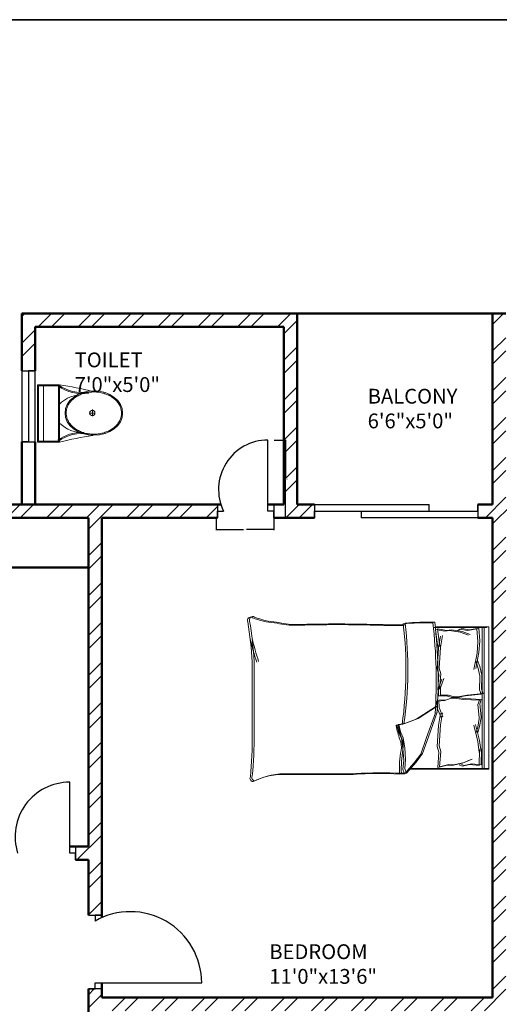
# Model space of a CAD drawing. Units: inches. Extents: x 963 to 2075, y 289 to 2657.
# Tile 81 of 98: x 1349 to 1511, y 2325 to 2657. Entities that reach past the tile are written whole.
import ezdxf

# ---------------------------------------------------------------- set-up
doc = ezdxf.new("R2010")
doc.units = ezdxf.units.IN
for name, color, linetype, lineweight in [('A-ANNO-DIMS', 2, 'Continuous', 18), ('A-ANNO-TTLB', 7, 'Continuous', 35), ('A-AREA-IDEN', 7, 'Continuous', 18), ('A-DOOR', 4, 'Continuous', 25), ('A-FLOR-FIXT', 9, 'Continuous', 18), ('A-FURN', 8, 'Continuous', 18), ('A-GLAZ', 3, 'Continuous', 25), ('A-WALL', 7, 'Continuous', 50), ('A-WALL-PATT', 8, 'Continuous', 13)]:
    doc.layers.add(name, color=color, linetype=linetype, lineweight=lineweight)
doc.styles.get("Standard").update_dxf_attribs({"font": 'arial.ttf'})
doc.dimstyles.get("Standard").update_dxf_attribs({"dimtxt": 0.18, "dimasz": 0.18, "dimexe": 0.18, "dimexo": 0.0625, "dimgap": 0.09, "dimtad": 0, "dimtih": 1, "dimtoh": 1, "dimdec": 4, "dimzin": 0, "dimdsep": 46, "dimtxsty": 'Standard', "dimcen": 0.09, "dimadec": 0, "dimazin": 0, "dimtfac": 1, "dimtdec": 4, "dimtofl": 0, "dimtmove": 0, "dimatfit": 3, "dimfxl": 1, "dimtolj": 1, "dimtzin": 0, "dimarcsym": 0})

# ---------------------------------------------------------------- blocks, each defined once
blk = doc.blocks.new('A$C31115884')
for p, q in [((283.1, 497.7), (223.4, 497.7)), ((257.5, 466.4), (257.5, 523.2)), ((0, 200), (0, 0)), ((520, 200), (0, 200)), ((10, 190), (10, 10)), ((510, 190), (10, 190)), ((510, 10), (510, 190)), ((520, 0), (520, 200)), ((510, 54.5), (0, 54.5)), ((10, 10), (510, 10)), ((0, 0), (520, 0))]:
    blk.add_line(p, q)
blk.add_circle((255.6, 496.4), 23.6)
for centre, radius, start, end in [((2777.7, -204.6), 2807, 165.4549, 171.71327), ((-294.5, 403.3), 364.7, 324.20913, 9.34987), ((-294.5, 403.3), 374.7, 324.20913, 9.34987), ((805.8, 403.3), 364.7, 170.65013, 215.79087), ((3237, 905), 2807, 188.28673, 194.5451), ((139.5, 406.2), 293.5, 315.84364, 2.65635), ((805.8, 403.3), 374.7, 179.20365, 215.79087), ((383.6, 406.2), 293.5, 190.27735, 224.15636)]:
    blk.add_arc(centre, radius, start, end)
blk.add_ellipse((256.2, 509.9), major_axis=(0, -260.7), ratio=0.772727)
blk.add_open_spline([(256.2, 259.2), (263.1, 259.2), (270, 259.7), (287.8, 262.3), (298.7, 265.1), (319.9, 273.1), (330.2, 278.4), (350.1, 291.1), (359.7, 298.7), (377.7, 315.9), (386.2, 325.5), (401.7, 346.6), (408.8, 358.1), (421.3, 382.5), (426.8, 395.5), (435.9, 422.4), (439.5, 436.4), (444.8, 465.1), (446.5, 479.7), (447.9, 509.2), (447.6, 524), (445, 553.3), (442.7, 567.8), (436.3, 596), (432.1, 609.7), (421.9, 636), (416, 648.6), (402.5, 672.1), (395, 683), (378.6, 703), (369.8, 712.1), (351.1, 728), (341.3, 734.8), (320.9, 746.2), (310.4, 750.7), (288.9, 757.3), (278, 759.4), (256, 761), (245, 760.6), (223.1, 757.2), (212.3, 754.3), (191.1, 746.1), (180.8, 740.7), (160.9, 727.8), (151.4, 720.1), (133.5, 702.7), (125.1, 693), (109.6, 671.7), (102.6, 660.2), (90.2, 635.7), (84.9, 622.7), (76, 595.6), (72.4, 581.6), (67.2, 552.9), (65.6, 538.2), (64.4, 508.8), (64.8, 494), (67.5, 464.7), (69.9, 450.2), (76.6, 422), (80.8, 408.3), (91.1, 382.2), (97.2, 369.7), (110.8, 346.3), (118.4, 335.4), (134.8, 315.6), (143.7, 306.7), (162.4, 290.9), (172.3, 284.2), (192.8, 273), (203.3, 268.6), (224.8, 262.2), (235.8, 260.2), (249.9, 259.3), (253, 259.2), (256.2, 259.2)], degree=3, knots=[0, 0, 0, 0, 0.110105, 0.110105, 0.285049, 0.285049, 0.459994, 0.459994, 0.634938, 0.634938, 0.809882, 0.809882, 0.984827, 0.984827, 1.159771, 1.159771, 1.334715, 1.334715, 1.50966, 1.50966, 1.684604, 1.684604, 1.859549, 1.859549, 2.034493, 2.034493, 2.209437, 2.209437, 2.384382, 2.384382, 2.559326, 2.559326, 2.73427, 2.73427, 2.909215, 2.909215, 3.084159, 3.084159, 3.259103, 3.259103, 3.434048, 3.434048, 3.608992, 3.608992, 3.783936, 3.783936, 3.958881, 3.958881, 4.133825, 4.133825, 4.30877, 4.30877, 4.483714, 4.483714, 4.658658, 4.658658, 4.833603, 4.833603, 5.008547, 5.008547, 5.183491, 5.183491, 5.358436, 5.358436, 5.53338, 5.53338, 5.708324, 5.708324, 5.883269, 5.883269, 6.058213, 6.058213, 6.233158, 6.233158, 6.283185, 6.283185, 6.283185, 6.283185])
blk = doc.blocks.new('BED-DOUBLE')
for p, q in [((1236.12, 2450.52), (1254.23, 2450.52)), ((1236.12, 2450.52), (1254.23, 2450.52)), ((1236.76, 2450.75), (1254.87, 2450.75)), ((1236.76, 2450.75), (1254.87, 2450.75)), ((1238.25, 2444.94), (1237.53, 2450.04)), ((1237.53, 2450.04), (1240.71, 2449.46)), ((1238.25, 2444.94), (1237.53, 2450.04)), ((1237.53, 2450.04), (1240.71, 2449.46)), ((1245.77, 2450.18), (1244.76, 2449.61)), ((1245.77, 2450.18), (1244.76, 2449.61)), ((1248.37, 2449.75), (1245.77, 2450.18)), ((1248.37, 2449.75), (1245.77, 2450.18)), ((1250.92, 2450.1), (1247.74, 2449.52)), ((1250.92, 2450.1), (1247.74, 2449.52)), ((1251.56, 2450.33), (1248.37, 2449.75)), ((1251.56, 2450.33), (1248.37, 2449.75)), ((1250.89, 2450.1), (1251.22, 2445.82)), ((1250.89, 2450.1), (1251.22, 2445.82)), ((1251.53, 2450.32), (1251.86, 2446.04)), ((1251.53, 2450.32), (1251.86, 2446.04)), ((1252.7, 2450.52), (1252.7, 2402.73)), ((1252.7, 2450.52), (1252.7, 2402.73)), ((1253.34, 2450.75), (1253.34, 2402.96)), ((1253.34, 2450.75), (1253.34, 2402.96)), ((1254.87, 2450.75), (1254.87, 2402.73)), ((1237.61, 2444.71), (1236.89, 2449.81)), ((1236.89, 2449.81), (1240.07, 2449.23)), ((1237.61, 2444.71), (1236.89, 2449.81)), ((1236.89, 2449.81), (1240.07, 2449.23)), ((1238.6, 2447.61), (1237.94, 2443.58)), ((1238.6, 2447.61), (1237.94, 2443.58)), ((1239.24, 2447.84), (1238.58, 2443.81)), ((1239.24, 2447.84), (1238.58, 2443.81)), ((1240.07, 2449.23), (1241.66, 2449.52)), ((1240.07, 2449.23), (1241.66, 2449.52)), ((1240.71, 2449.46), (1242.3, 2449.75)), ((1240.71, 2449.46), (1242.3, 2449.75)), ((1241.66, 2449.52), (1245.28, 2448.94)), ((1241.66, 2449.52), (1245.28, 2448.94)), ((1242.3, 2449.75), (1245.92, 2449.17)), ((1242.3, 2449.75), (1245.92, 2449.17)), ((1245.13, 2449.96), (1244.12, 2449.38)), ((1245.13, 2449.96), (1244.12, 2449.38)), ((1247.74, 2449.52), (1245.13, 2449.96)), ((1247.74, 2449.52), (1245.13, 2449.96)), ((1245.28, 2448.94), (1248.02, 2447.93)), ((1245.28, 2448.94), (1248.02, 2447.93)), ((1245.92, 2449.17), (1248.66, 2448.16)), ((1245.92, 2449.17), (1248.66, 2448.16)), ((1237.94, 2443.58), (1237.51, 2436.57)), ((1237.94, 2443.58), (1237.51, 2436.57)), ((1237.94, 2443.58), (1237.61, 2444.71)), ((1237.94, 2443.58), (1237.61, 2444.71)), ((1238.58, 2443.81), (1238.15, 2436.8)), ((1238.58, 2443.81), (1238.15, 2436.8)), ((1238.58, 2443.81), (1238.25, 2444.94)), ((1238.58, 2443.81), (1238.25, 2444.94)), ((1251.21, 2445.71), (1250.92, 2441.89)), ((1251.21, 2445.71), (1250.92, 2441.89)), ((1251.22, 2445.82), (1251.21, 2445.71)), ((1251.22, 2445.82), (1251.21, 2445.71)), ((1251.84, 2445.94), (1251.56, 2442.11)), ((1251.84, 2445.94), (1251.56, 2442.11)), ((1251.86, 2446.04), (1251.84, 2445.94)), ((1251.86, 2446.04), (1251.84, 2445.94)), ((1250.92, 2441.89), (1249.9, 2436.39)), ((1250.92, 2441.89), (1249.9, 2436.39)), ((1251.56, 2442.11), (1250.54, 2436.62)), ((1251.56, 2442.11), (1250.54, 2436.62)), ((1174.99, 2438.93), (1174.99, 2414.32)), ((1174.99, 2438.93), (1174.99, 2414.32)), ((1175.63, 2439.16), (1175.63, 2414.55)), ((1175.63, 2439.16), (1175.63, 2414.55)), ((1238.15, 2436.8), (1238.7, 2434.84)), ((1238.15, 2436.8), (1238.7, 2434.84)), ((1250.48, 2439.14), (1251.21, 2437.12)), ((1250.48, 2439.14), (1251.21, 2437.12)), ((1251.12, 2439.37), (1251.84, 2437.34)), ((1251.12, 2439.37), (1251.84, 2437.34)), ((1251.21, 2437.12), (1251.93, 2434.22)), ((1251.21, 2437.12), (1251.93, 2434.23)), ((1251.84, 2437.34), (1252.57, 2434.45)), ((1251.84, 2437.34), (1252.57, 2434.45)), ((1237.51, 2436.57), (1238.06, 2434.61)), ((1237.51, 2436.57), (1238.06, 2434.61)), ((1238.06, 2434.61), (1237.66, 2429.48)), ((1238.06, 2434.61), (1237.66, 2429.48)), ((1238.7, 2434.84), (1238.3, 2429.71)), ((1238.7, 2434.84), (1238.3, 2429.71)), ((1251.93, 2433.9), (1251.78, 2429.46)), ((1251.93, 2433.9), (1251.78, 2429.46)), ((1251.93, 2434.23), (1251.93, 2433.9)), ((1251.93, 2434.22), (1251.93, 2433.9)), ((1252.57, 2434.13), (1252.42, 2429.69)), ((1252.57, 2434.13), (1252.42, 2429.69)), ((1252.57, 2434.45), (1252.57, 2434.13)), ((1252.57, 2434.45), (1252.57, 2434.13)), ((1237.97, 2429.89), (1239.06, 2433.04)), ((1237.97, 2429.89), (1239.06, 2433.04)), ((1238.61, 2430.12), (1239.7, 2433.26)), ((1238.61, 2430.12), (1239.7, 2433.26)), ((1238.61, 2427.66), (1238.61, 2430.12)), ((1238.61, 2427.66), (1238.61, 2430.12)), ((1237.97, 2427.43), (1237.97, 2429.89)), ((1237.97, 2427.43), (1237.97, 2429.89)), ((1240.65, 2427.43), (1237.97, 2427.43)), ((1240.65, 2427.43), (1237.97, 2427.43)), ((1241.29, 2427.66), (1238.61, 2427.66)), ((1241.29, 2427.66), (1238.61, 2427.66)), ((1242.53, 2426.86), (1240.65, 2427.43)), ((1242.53, 2426.86), (1240.65, 2427.43)), ((1242.49, 2426.79), (1240.66, 2426.09)), ((1242.49, 2426.79), (1240.66, 2426.09)), ((1243.17, 2427.08), (1241.29, 2427.66)), ((1243.17, 2427.08), (1241.29, 2427.66)), ((1243.79, 2426.87), (1242.49, 2426.79)), ((1243.79, 2426.87), (1242.49, 2426.79)), ((1243.83, 2426.86), (1242.53, 2426.86)), ((1243.83, 2426.86), (1242.53, 2426.86)), ((1244.47, 2427.08), (1243.17, 2427.08)), ((1244.47, 2427.08), (1243.17, 2427.08)), ((1247, 2426.49), (1243.79, 2426.87)), ((1247, 2426.49), (1243.79, 2426.87)), ((1247.01, 2427.43), (1243.83, 2426.86)), ((1247.01, 2427.43), (1243.83, 2426.86)), ((1247.65, 2427.66), (1244.47, 2427.08)), ((1247.65, 2427.66), (1244.47, 2427.08)), ((1252.36, 2428.01), (1247.01, 2427.43)), ((1252.36, 2428.01), (1247.01, 2427.43)), ((1253, 2428.24), (1247.65, 2427.66)), ((1253, 2428.24), (1247.65, 2427.66)), ((1251.78, 2429.46), (1252.36, 2428.01)), ((1251.78, 2429.46), (1252.36, 2428.01)), ((1252.42, 2429.69), (1253, 2428.24)), ((1252.42, 2429.69), (1253, 2428.24)), ((1236.85, 2423.74), (1230.36, 2419.55)), ((1236.85, 2423.74), (1230.36, 2419.55)), ((1237.49, 2423.96), (1231, 2419.77)), ((1237.49, 2423.96), (1231, 2419.77)), ((1240.02, 2425.86), (1237.34, 2425.7)), ((1240.02, 2425.86), (1237.34, 2425.7)), ((1237.34, 2425.7), (1237.49, 2423.24)), ((1237.34, 2425.7), (1237.49, 2423.24)), ((1240.66, 2426.09), (1237.98, 2425.93)), ((1240.66, 2426.09), (1237.98, 2425.93)), ((1237.98, 2425.93), (1238.13, 2423.47)), ((1237.98, 2425.93), (1238.13, 2423.47)), ((1238.13, 2423.47), (1239.42, 2420.4)), ((1238.13, 2423.47), (1239.42, 2420.4)), ((1241.86, 2426.56), (1240.02, 2425.86)), ((1241.86, 2426.56), (1240.02, 2425.86)), ((1243.15, 2426.64), (1241.86, 2426.56)), ((1243.15, 2426.64), (1241.86, 2426.56)), ((1246.37, 2426.26), (1243.15, 2426.64)), ((1246.37, 2426.26), (1243.15, 2426.64)), ((1251.74, 2426.02), (1246.37, 2426.26)), ((1251.74, 2426.02), (1246.37, 2426.26)), ((1252.38, 2426.25), (1247, 2426.49)), ((1252.38, 2426.25), (1247, 2426.49)), ((1251.25, 2424.54), (1251.74, 2426.02)), ((1251.25, 2424.54), (1251.74, 2426.02)), ((1251.68, 2420.11), (1251.25, 2424.54)), ((1251.68, 2420.11), (1251.25, 2424.54)), ((1251.89, 2424.77), (1252.38, 2426.25)), ((1251.89, 2424.77), (1252.38, 2426.25)), ((1252.31, 2420.34), (1251.89, 2424.77)), ((1252.31, 2420.34), (1251.89, 2424.77)), ((1233.92, 2413.35), (1236.85, 2421.69)), ((1233.92, 2413.35), (1236.85, 2421.69)), ((1234.56, 2413.58), (1237.49, 2421.92)), ((1234.56, 2413.58), (1237.49, 2421.92)), ((1237.49, 2423.24), (1238.78, 2420.17)), ((1237.49, 2423.24), (1238.78, 2420.17)), ((1238.6, 2421.43), (1237.94, 2417.4)), ((1238.6, 2421.43), (1237.94, 2417.4)), ((1239.24, 2421.66), (1238.58, 2417.63)), ((1239.24, 2421.66), (1238.58, 2417.63)), ((1251.7, 2419.79), (1251.68, 2420.11)), ((1251.7, 2419.79), (1251.68, 2420.11)), ((1252.33, 2420.02), (1252.31, 2420.34)), ((1252.33, 2420.02), (1252.31, 2420.34)), ((1225.87, 2417.84), (1223.86, 2417.53)), ((1225.87, 2417.84), (1223.86, 2417.53)), ((1223.86, 2417.53), (1224.47, 2415.05)), ((1223.86, 2417.53), (1224.47, 2415.05)), ((1226.51, 2418.07), (1224.49, 2417.76)), ((1226.51, 2418.07), (1224.49, 2417.76)), ((1224.49, 2417.76), (1225.11, 2415.28)), ((1224.49, 2417.76), (1225.11, 2415.28)), ((1230.36, 2419.55), (1225.87, 2417.84)), ((1230.36, 2419.55), (1225.87, 2417.84)), ((1231, 2419.77), (1226.51, 2418.07)), ((1231, 2419.77), (1226.51, 2418.07)), ((1237.94, 2417.4), (1237.51, 2410.39)), ((1237.94, 2417.4), (1237.51, 2410.39)), ((1238.58, 2417.63), (1238.15, 2410.62)), ((1238.58, 2417.63), (1238.15, 2410.62)), ((1251.16, 2412.08), (1249.81, 2417.5)), ((1251.16, 2412.08), (1249.81, 2417.5)), ((1251.8, 2412.31), (1250.45, 2417.73)), ((1251.8, 2412.31), (1250.45, 2417.73)), ((1250.56, 2414.79), (1251.15, 2416.86)), ((1250.56, 2414.79), (1251.15, 2416.86)), ((1251.15, 2416.86), (1251.7, 2419.79)), ((1251.15, 2416.86), (1251.7, 2419.79)), ((1251.2, 2415.02), (1251.79, 2417.09)), ((1251.2, 2415.02), (1251.79, 2417.09)), ((1251.79, 2417.09), (1252.33, 2420.02)), ((1251.79, 2417.09), (1252.33, 2420.02)), ((1224.47, 2415.05), (1225.4, 2413.04)), ((1224.47, 2415.05), (1225.4, 2413.04)), ((1225.11, 2415.28), (1226.04, 2413.27)), ((1225.11, 2415.28), (1226.04, 2413.27)), ((1232.54, 2408), (1234.56, 2413.58)), ((1232.54, 2408), (1234.56, 2413.58)), ((1225.4, 2413.04), (1225.87, 2409.63)), ((1225.4, 2413.04), (1225.87, 2409.63)), ((1226.04, 2413.27), (1226.51, 2409.86)), ((1226.04, 2413.27), (1226.51, 2409.86)), ((1231.9, 2407.77), (1233.92, 2413.35)), ((1231.9, 2407.78), (1233.92, 2413.35)), ((1237.51, 2410.39), (1238.06, 2408.43)), ((1237.51, 2410.39), (1238.06, 2408.43)), ((1238.15, 2410.62), (1238.7, 2408.66)), ((1238.15, 2410.62), (1238.7, 2408.66)), ((1251.69, 2408.28), (1251.16, 2412.08)), ((1251.69, 2408.28), (1251.16, 2412.08)), ((1252.33, 2408.51), (1251.8, 2412.31)), ((1252.33, 2408.51), (1251.8, 2412.31)), ((1225.87, 2409.63), (1226.18, 2405.76)), ((1225.87, 2409.63), (1226.18, 2405.76)), ((1226.51, 2409.86), (1226.82, 2405.99)), ((1226.51, 2409.86), (1226.82, 2405.99)), ((1229.74, 2404.83), (1231.9, 2407.78)), ((1229.74, 2404.83), (1231.9, 2407.77)), ((1230.38, 2405.06), (1232.54, 2408)), ((1230.38, 2405.06), (1232.54, 2408)), ((1238.06, 2408.43), (1237.66, 2403.3)), ((1238.06, 2408.43), (1237.66, 2403.3)), ((1238.7, 2408.66), (1238.3, 2403.52)), ((1238.7, 2408.66), (1238.3, 2403.52)), ((1251.68, 2403.88), (1251.77, 2409.29)), ((1251.68, 2403.88), (1251.77, 2409.28)), ((1251.77, 2409.29), (1251.69, 2408.28)), ((1251.77, 2409.28), (1251.69, 2408.28)), ((1252.31, 2404.11), (1252.41, 2409.51)), ((1252.31, 2404.11), (1252.41, 2409.51)), ((1252.41, 2409.51), (1252.33, 2408.51)), ((1252.41, 2409.51), (1252.33, 2408.51)), ((1226.18, 2405.76), (1225.87, 2402.66)), ((1226.18, 2405.76), (1225.87, 2402.66)), ((1226.49, 2401.13), (1229.74, 2404.83)), ((1226.49, 2401.13), (1229.74, 2404.83)), ((1226.82, 2405.99), (1226.51, 2402.89)), ((1226.82, 2405.99), (1226.51, 2402.89)), ((1227.13, 2401.36), (1230.38, 2405.06)), ((1227.13, 2401.36), (1230.38, 2405.06)), ((1237.66, 2403.3), (1240.8, 2404.07)), ((1237.66, 2403.3), (1240.8, 2404.07)), ((1238.3, 2403.52), (1241.44, 2404.3)), ((1238.3, 2403.52), (1241.44, 2404.3)), ((1240.8, 2404.07), (1242.4, 2403.88)), ((1240.8, 2404.07), (1242.4, 2403.88)), ((1241.44, 2404.3), (1243.04, 2404.11)), ((1241.44, 2404.3), (1243.04, 2404.11)), ((1242.4, 2403.88), (1245.98, 2404.69)), ((1242.4, 2403.88), (1245.98, 2404.69)), ((1243.04, 2404.11), (1246.61, 2404.91)), ((1243.04, 2404.11), (1246.61, 2404.91)), ((1245.89, 2403.67), (1244.85, 2404.18)), ((1245.89, 2403.67), (1244.85, 2404.18)), ((1246.53, 2403.89), (1245.49, 2404.41)), ((1246.53, 2403.89), (1245.49, 2404.41)), ((1248.46, 2404.26), (1245.89, 2403.67)), ((1248.46, 2404.26), (1245.89, 2403.67)), ((1245.98, 2404.69), (1248.65, 2405.87)), ((1245.98, 2404.69), (1248.65, 2405.87)), ((1249.1, 2404.49), (1246.53, 2403.89)), ((1249.1, 2404.49), (1246.53, 2403.89)), ((1246.61, 2404.91), (1249.29, 2406.1)), ((1246.61, 2404.91), (1249.29, 2406.09)), ((1251.68, 2403.88), (1248.46, 2404.26)), ((1251.68, 2403.88), (1248.46, 2404.26)), ((1252.31, 2404.11), (1249.1, 2404.49)), ((1252.31, 2404.11), (1249.1, 2404.49)), ((1224.74, 2401.05), (1226.49, 2401.13, 3.87)), ((1224.74, 2401.05), (1226.49, 2401.13, 3.87)), ((1225.38, 2401.28), (1227.13, 2401.36, 3.87)), ((1225.38, 2401.28), (1227.13, 2401.36, 3.87)), ((1225.87, 2402.66), (1226.49, 2401.13)), ((1225.87, 2402.66), (1226.49, 2401.13)), ((1226.51, 2402.89), (1227.13, 2401.36)), ((1226.51, 2402.89), (1227.13, 2401.36)), ((1254.23, 2402.73), (1227.62, 2402.73)), ((1254.23, 2402.73), (1227.62, 2402.73)), ((1254.87, 2402.96), (1228.26, 2402.96)), ((1254.87, 2402.96), (1228.26, 2402.96)), ((1254.87, 2402.73), (1254.23, 2402.73))]:
    blk.add_line(p, q)
for centre, radius, start, end in [((1174.51, 2452.91), 1.09, 56.1736, 203.4781), ((1174.51, 2452.91), 1.09, 56.1736, 203.4781), ((1175.15, 2453.14), 1.09, 56.1736, 203.4781), ((1175.15, 2453.14), 1.09, 56.1736, 203.4781), ((1183.96, 2475.65), 23.56, 247.9751, 266.652), ((1183.96, 2475.65), 23.56, 247.9751, 266.652), ((1184.6, 2475.88), 23.56, 247.9751, 266.652), ((1184.6, 2475.88), 23.56, 247.9751, 266.652), ((1053.4, 2432.57), 121.76, 2.9958, 9.4091), ((1053.4, 2432.57), 121.76, 2.9958, 9.4091), ((1054.03, 2432.8), 121.76, 2.9958, 9.4091), ((1054.03, 2432.8), 121.76, 2.9958, 9.4091), ((1189.72, 2480.89), 29.63, 256.0648, 268.9113), ((1189.72, 2480.89), 29.63, 256.0648, 268.9113), ((1190.36, 2481.12), 29.63, 256.0648, 268.9113), ((1190.36, 2481.12), 29.63, 256.0648, 268.9113), ((1203.62, 1969.17), 482.31, 88.2277, 91.7185), ((1203.62, 1969.17), 482.31, 88.2277, 91.7185), ((1204.26, 1969.4), 482.31, 88.2277, 91.7185), ((1204.26, 1969.4), 482.31, 88.2277, 91.7185), ((1223.06, 2621.3), 170.11, 268.4762, 271.0082), ((1223.06, 2621.3), 170.11, 268.4762, 271.0082), ((1223.7, 2621.53), 170.11, 268.4762, 271.0082), ((1223.7, 2621.53), 170.11, 268.4762, 271.0082), ((1097.92, 2436.24), 129.02, 351.7845, 6.9006), ((1097.92, 2436.24), 129.02, 351.7845, 6.9006), ((1234.14, 2368.83), 83.31, 88.7218, 95.604), ((1234.14, 2368.83), 83.31, 88.7218, 95.604), ((1098.56, 2436.47), 129.02, 351.7845, 6.9006), ((1098.56, 2436.47), 129.02, 351.7845, 6.9006), ((1234.78, 2369.06), 83.31, 88.7218, 95.604), ((1234.78, 2369.06), 83.31, 88.7218, 95.604), ((1072.18, 2432.64), 164.97, 356.0865, 6.7821), ((1072.18, 2432.64), 164.97, 356.0865, 6.7821), ((1072.82, 2432.86), 164.97, 356.0865, 6.7821), ((1072.82, 2432.86), 164.97, 356.0865, 6.7821), ((1278.58, 2471.44), 106.46, 193.3832, 197.7053), ((1278.58, 2471.44), 106.46, 193.3832, 197.7053), ((1277.94, 2471.22), 106.46, 193.3832, 197.7053), ((1277.94, 2471.22), 106.46, 193.3832, 197.7053), ((1223.79, 2417.36), 0.185, 70.2464, 181.1377), ((1223.79, 2417.36), 0.185, 70.2464, 181.1377), ((1252.75, 2422.84), 29.65, 190.6617, 199.8806), ((1252.75, 2422.84), 29.65, 190.6617, 199.8806), ((1224.43, 2417.59), 0.185, 70.2464, 181.1377), ((1224.43, 2417.59), 0.185, 70.2464, 181.1377), ((1253.39, 2423.07), 29.65, 190.6617, 199.8806), ((1253.39, 2423.07), 29.65, 190.6617, 199.8806), ((1041.96, 2412.84), 133.04, 354.4998, 0.6351), ((1041.96, 2412.84), 133.04, 354.4998, 0.6351), ((1042.6, 2413.07), 133.04, 354.4998, 0.6351), ((1042.6, 2413.07), 133.04, 354.4998, 0.6351), ((1219.17, 2410.25), 6.22, 348.6608, 23.7384), ((1219.17, 2410.25), 6.22, 348.6608, 23.7384), ((1219.81, 2410.48), 6.22, 348.6608, 23.7384), ((1219.81, 2410.48), 6.22, 348.6608, 23.7384), ((1260.89, 2402.67), 36.18, 169.8763, 182.5657), ((1260.89, 2402.67), 36.18, 169.8763, 182.5657), ((1261.53, 2402.9), 36.18, 169.8763, 182.5657), ((1261.53, 2402.9), 36.18, 169.8763, 182.5657), ((1176, 2399.81), 1.1, 152.6588, 266.02), ((1176, 2399.81), 1.1, 152.6588, 266.02), ((1185.57, 2377.84), 23.07, 87.4714, 116.4681), ((1185.57, 2377.84), 23.07, 87.4714, 116.4681), ((1186.21, 2378.07), 23.07, 87.4714, 116.4681), ((1186.21, 2378.07), 23.07, 87.4714, 116.4681), ((1186.41, 6962.74), 4561.86, 270.00217, 270.28689), ((1186.41, 6962.74), 4561.86, 270.00217, 270.28689), ((1187.05, 6962.97), 4561.86, 270.00217, 270.28689), ((1187.05, 6962.97), 4561.86, 270.00217, 270.28689), ((1217.92, 2271.73), 129.5, 86.9791, 93.8365), ((1217.92, 2271.73), 129.5, 86.9791, 93.8365), ((1218.56, 2271.96), 129.5, 86.9791, 93.8365), ((1218.56, 2271.96), 129.5, 86.9791, 93.8365), ((1175.36, 2399.58), 1.1, 152.6588, 266.02), ((1175.36, 2399.58), 1.1, 152.6588, 266.02)]:
    blk.add_arc(centre, radius, start, end)
blk = doc.blocks.new('DOOR-4')
for p, q in [((16.99, 2.25), (16.99, 26.25)), ((0, 4.5), (0, 0)), ((18.99, 4.5), (18.99, 0)), ((0, 0), (0, 2.25)), ((0, 2.25), (2, 2.25)), ((18.99, 2.25), (16.99, 2.25)), ((18.99, 0), (18.99, 2.25))]:
    blk.add_line(p, q)
blk.add_arc((16.99, 9.57), 16.68, 90, 206.0308)
blk = doc.blocks.new('*D36')
at = {"layer": 'A-ANNO-DIMS', "color": 0, "lineweight": -2, "transparency": 16777216}
for p, q in [((1434.6, 2515.57), (1438.66, 2515.57)), ((1438.48, 2515.39), (1438.48, 2502.63)), ((1438.48, 2489.5), (1438.48, 2502.26)), ((1434.6, 2489.32), (1438.66, 2489.32))]:
    blk.add_line(p, q, dxfattribs=at)
at = {"layer": 'A-ANNO-DIMS', "color": 0, "transparency": 16777216}
for points in [[(1438.45, 2515.39), (1438.51, 2515.39), (1438.48, 2515.57)], [(1438.45, 2489.5), (1438.51, 2489.5), (1438.48, 2489.32)]]:
    blk.add_solid(points, dxfattribs=at)
at = {"layer": 'Defpoints', "color": 0, "transparency": 16777216}
for p in [(1434.54, 2515.57), (1438.48, 2515.57), (1434.54, 2489.32)]:
    blk.add_point(p, dxfattribs=at)
at = {"layer": 'A-ANNO-DIMS', "color": 0, "transparency": 16777216, "insert": (1438.48, 2502.44), "char_height": 0.18, "attachment_point": 5}
blk.add_mtext('\\A1;DOOR D4 26 TYP.', dxfattribs=at)
blk = doc.blocks.new('*D37')
at = {"layer": 'A-ANNO-DIMS', "color": 0, "lineweight": -2, "transparency": 16777216}
for p, q in [((1415.03, 2489.26), (1415.03, 2485.2)), ((1434.54, 2489.26), (1434.54, 2485.2)), ((1415.21, 2485.38), (1424.26, 2485.38)), ((1434.36, 2485.38), (1425.32, 2485.38))]:
    blk.add_line(p, q, dxfattribs=at)
at = {"layer": 'A-ANNO-DIMS', "color": 0, "transparency": 16777216}
for points in [[(1415.21, 2485.41), (1415.21, 2485.35), (1415.03, 2485.38)], [(1434.36, 2485.41), (1434.36, 2485.35), (1434.54, 2485.38)]]:
    blk.add_solid(points, dxfattribs=at)
at = {"layer": 'Defpoints', "color": 0, "transparency": 16777216}
for p in [(1415.03, 2489.32), (1434.54, 2489.32), (1434.54, 2485.38)]:
    blk.add_point(p, dxfattribs=at)
at = {"layer": 'A-ANNO-DIMS', "color": 0, "transparency": 16777216, "insert": (1424.79, 2485.38), "char_height": 0.18, "attachment_point": 5}
blk.add_mtext('\\A1;20 TYP.', dxfattribs=at)

msp = doc.modelspace()

# ---------------------------------------------------------------- hatches: boundary and pattern name
at = {"layer": 'A-WALL-PATT'}
h = msp.add_hatch(dxfattribs=at)
h.set_pattern_fill('ANSI32', color=256)
h.paths.add_polyline_path([(1296.92, 2558.32), (1203.92, 2558.32), (1203.92, 2493.82), (1191.53, 2493.82), (1191.53, 2489.32), (1211.06, 2489.32), (1211.06, 2492.02), (1211.06, 2493.82), (1208.42, 2493.82), (1208.42, 2553.82), (1292.42, 2553.82), (1292.42, 2538.86), (1296.92, 2538.86)])
h.paths.add_polyline_path([(1442.42, 2558.32), (1349.42, 2558.32), (1349.42, 2538.94), (1353.92, 2538.94), (1353.92, 2553.82), (1437.92, 2553.82), (1437.92, 2493.82), (1434.54, 2493.82), (1434.54, 2489.32), (1448.31, 2489.32), (1448.31, 2491.57), (1448.31, 2493.82), (1442.42, 2493.82)])
h.paths.add_polyline_path([(1415.55, 2491.57), (1415.55, 2493.82), (1340.94, 2493.82), (1340.94, 2489.32), (1371.92, 2489.32), (1371.92, 2378.32), (1367.6, 2378.32), (1367.6, 2373.82), (1371.92, 2373.82), (1371.92, 2355.19), (1376.42, 2355.19), (1376.42, 2489.32), (1415.55, 2489.32)])
h.paths.add_polyline_path([(1304.94, 2491.57), (1304.94, 2493.82), (1296.92, 2493.82), (1296.92, 2514.86), (1292.42, 2514.86), (1292.42, 2493.82), (1232.81, 2493.82), (1232.81, 2489.32), (1256.42, 2489.32), (1256.42, 2327.32), (1253.71, 2327.32), (1253.71, 2322.82), (1328.42, 2322.82), (1328.42, 2331.15), (1323.92, 2331.15), (1323.92, 2327.32), (1260.92, 2327.32), (1260.92, 2373.82), (1323.92, 2373.82), (1323.92, 2357.81), (1328.42, 2357.81), (1328.42, 2373.82), (1346.01, 2373.82), (1346.01, 2376.07), (1346.01, 2378.32), (1260.92, 2378.32), (1260.92, 2489.32), (1304.94, 2489.32)])
h.paths.add_polyline_path([(1226.65, 2327.32), (1124.42, 2327.32), (1124.42, 2347.45), (1119.92, 2347.45), (1119.92, 2322.82), (1163.42, 2322.82), (1163.42, 2305.43), (1165.67, 2305.43), (1167.92, 2305.43), (1167.92, 2322.82), (1226.65, 2322.82), (1226.65, 2325.07)])
h.paths.add_polyline_path([(1095.92, 2489.32), (1124.42, 2489.32), (1131.53, 2489.32), (1131.53, 2491.57), (1131.53, 2493.82), (1119.92, 2493.82), (1091.42, 2493.82), (1091.42, 2417.32), (1095.92, 2417.32), (1119.92, 2417.32), (1119.92, 2407.45), (1124.42, 2407.45), (1124.42, 2421.82), (1095.92, 2421.82)])
h.paths.add_polyline_path([(1512.92, 2558.32), (1508.42, 2558.32), (1508.42, 2493.82), (1503.4, 2493.82), (1503.4, 2489.32), (1508.42, 2489.32), (1508.42, 2327.32), (1376.42, 2327.32), (1376.42, 2330.27), (1371.92, 2330.27), (1371.92, 2298.74), (1376.42, 2298.74), (1376.42, 2322.82), (1508.42, 2322.82), (1508.42, 2165.32), (1504.26, 2165.32), (1504.26, 2160.82), (1508.42, 2160.82), (1508.42, 2108.32), (1512.92, 2108.32), (1512.92, 2160.82), (1516.18, 2160.82), (1516.18, 2163.07), (1516.18, 2165.32), (1512.92, 2165.32), (1512.92, 2322.82), (1644.92, 2322.82), (1644.92, 2298.74), (1649.42, 2298.74), (1649.42, 2322.82), (1649.42, 2330.94), (1647.17, 2330.94), (1644.92, 2330.94), (1644.92, 2327.32), (1512.92, 2327.32), (1512.92, 2489.32), (1516.76, 2489.32), (1516.76, 2491.57), (1516.76, 2493.82), (1512.92, 2493.82)])
h.paths.add_polyline_path([(1671.92, 2558.32), (1578.92, 2558.32), (1578.92, 2493.82), (1573.53, 2493.82), (1573.53, 2489.32), (1586.54, 2489.32), (1586.54, 2491.57), (1586.54, 2493.82), (1583.42, 2493.82), (1583.42, 2553.82), (1667.42, 2553.82), (1667.42, 2541.11), (1671.92, 2541.11)])
h.paths.add_polyline_path([(1681.26, 2493.82), (1671.92, 2493.82), (1671.92, 2517.11), (1667.42, 2517.11), (1667.42, 2493.82), (1610.22, 2493.82), (1610.22, 2489.32), (1644.92, 2489.32), (1644.92, 2357.87), (1649.42, 2357.87), (1649.42, 2373.82), (1652.2, 2373.82), (1652.2, 2375.83), (1652.2, 2378.32), (1649.42, 2378.32), (1649.42, 2489.32), (1681.26, 2489.32), (1681.26, 2491.57)])
h.paths.add_polyline_path([(1821.92, 2558.32), (1728.92, 2558.32), (1728.92, 2541), (1733.42, 2541), (1733.42, 2553.82), (1817.42, 2553.82), (1817.42, 2493.82), (1813.51, 2493.82), (1813.51, 2489.32), (1830.08, 2489.32), (1830.08, 2491.57), (1830.08, 2493.82), (1821.92, 2493.82)])
h.paths.add_polyline_path([(1794.24, 2493.82), (1717.26, 2493.82), (1717.26, 2489.32), (1760.42, 2489.32), (1760.42, 2378.32), (1674.4, 2378.32), (1674.4, 2373.82), (1692.92, 2373.82), (1692.92, 2356.95), (1697.42, 2356.95), (1697.42, 2373.82), (1760.42, 2373.82), (1760.42, 2327.32), (1697.42, 2327.32), (1697.42, 2333.34), (1692.92, 2333.34), (1692.92, 2322.82), (1768.04, 2322.82), (1768.04, 2325.07), (1768.04, 2327.32), (1764.92, 2327.32), (1764.92, 2489.32), (1794.24, 2489.32)])
h.paths.add_polyline_path([(1733.42, 2517), (1728.92, 2517), (1728.92, 2493.82), (1733.42, 2493.82)], flags=17)
h.paths.add_polyline_path([(1929.92, 2493.82), (1890.08, 2493.82), (1890.08, 2489.32), (1896.92, 2489.32), (1925.42, 2489.32), (1925.42, 2421.82), (1896.92, 2421.82), (1896.92, 2408.32), (1901.42, 2408.32), (1901.42, 2417.32), (1925.42, 2417.32), (1929.92, 2417.32)])
h.paths.add_polyline_path([(1901.42, 2348.32), (1896.92, 2348.32), (1896.92, 2327.32), (1800.42, 2327.32), (1800.42, 2322.82), (1853.42, 2322.82), (1853.42, 2309.45), (1857.92, 2309.45), (1857.92, 2322.82), (1901.42, 2322.82)])
h.paths.add_polyline_path([(1857.92, 2249.45), (1853.42, 2249.45), (1853.42, 2214.82), (1686.31, 2214.82), (1686.31, 2210.32), (1853.42, 2210.32), (1853.42, 2202.13), (1857.92, 2202.13), (1857.92, 2210.32)])
h.paths.add_polyline_path([(1857.92, 2142.13), (1853.42, 2142.13), (1853.42, 2115.42), (1841.42, 2115.42), (1841.42, 2088.53), (1841.42, 2046.95), (1845.92, 2046.95), (1845.92, 2110.92), (1905.92, 2110.92), (1905.92, 2092.52), (1910.42, 2092.52), (1910.42, 2115.42), (1857.92, 2115.42)])
h.paths.add_polyline_path([(1532.44, 1482.34), (1573.46, 1482.34), (1573.46, 1501), (1532.44, 1501)], flags=9)
h.paths.add_polyline_path([(1438.66, 1486.3), (1479.68, 1486.3), (1479.68, 1504.96), (1438.66, 1504.96)], flags=9)
h.paths.add_polyline_path([(1411.22, 1365.31), (1659.14, 1365.31), (1659.14, 1402.4), (1411.22, 1402.4)], flags=9)
h.paths.add_polyline_path([(1185.67, 2296.3), (1248.16, 2296.3), (1248.16, 2314.95), (1185.67, 2314.95)], flags=9)
h.paths.add_polyline_path([(1177.31, 2187.35), (1216.15, 2187.35), (1216.15, 2206.01), (1177.31, 2206.01)], flags=9)
h.paths.add_polyline_path([(1295.1, 1602.08), (1328.26, 1602.08), (1328.26, 1620.74), (1295.1, 1620.74)], flags=9)
h.paths.add_polyline_path([(1525.13, 2005.99), (1558.39, 2005.99), (1558.39, 2024.65), (1525.13, 2024.65)], flags=9)
h.paths.add_polyline_path([(1459.61, 1977.13), (1472.19, 1977.13), (1472.19, 1987.43), (1459.61, 1987.43)], flags=9)
h.paths.add_polyline_path([(1467.81, 2053.68), (1480.02, 2053.68), (1480.02, 2063.98), (1467.81, 2063.98)], flags=9)
h.paths.add_polyline_path([(1555.18, 2119.02), (1584.56, 2119.02), (1584.56, 2137.68), (1555.18, 2137.68)], flags=25)
h.paths.add_polyline_path([(1405.39, 2115.29), (1444.48, 2115.29), (1444.48, 2133.95), (1405.39, 2133.95)], flags=25)
h.paths.add_polyline_path([(1698.48, 2004.26), (1727.69, 2004.26), (1727.69, 2022.92), (1698.48, 2022.92)], flags=9)
h.paths.add_polyline_path([(1612.16, 1972.86), (1629.02, 1972.86), (1629.02, 1983.16), (1612.16, 1983.16)], flags=9)
h.paths.add_polyline_path([(1608.29, 2060.04), (1625.15, 2060.04), (1625.15, 2070.34), (1608.29, 2070.34)], flags=9)
h.paths.add_polyline_path([(1527.95, 1684.4), (1566.79, 1684.4), (1566.79, 1703.06), (1527.95, 1703.06)], flags=9)
h.paths.add_polyline_path([(1422.79, 1683.59), (1461.63, 1683.59), (1461.63, 1702.25), (1422.79, 1702.25)], flags=9)
h.paths.add_polyline_path([(1531.26, 1732.46), (1574.01, 1732.46), (1574.01, 1751.12), (1531.26, 1751.12)], flags=9)
h.paths.add_polyline_path([(1402.87, 1732.85), (1439.8, 1732.85), (1439.8, 1751.5), (1402.87, 1751.5)], flags=9)
h.paths.add_polyline_path([(1243.12, 1923.13), (1281.96, 1923.13), (1281.96, 1941.79), (1243.12, 1941.79)], flags=9)
h.paths.add_polyline_path([(1181.75, 1792.27), (1244.24, 1792.27), (1244.24, 1810.93), (1181.75, 1810.93)], flags=9)
h.paths.add_polyline_path([(1265.82, 1670.3), (1316.07, 1670.3), (1316.07, 1688.96), (1265.82, 1688.96)], flags=9)
h.paths.add_polyline_path([(1140.26, 1676.05), (1179.1, 1676.05), (1179.1, 1694.71), (1140.26, 1694.71)], flags=9)
h.paths.add_polyline_path([(1107.49, 1490.89), (1143.37, 1490.89), (1143.37, 1509.55), (1107.49, 1509.55)], flags=9)
h.paths.add_polyline_path([(1217.58, 1483.9), (1246.74, 1483.9), (1246.74, 1502.56), (1217.58, 1502.56)], flags=9)
h.paths.add_polyline_path([(1389.21, 1486.92), (1418.37, 1486.92), (1418.37, 1505.58), (1389.21, 1505.58)], flags=9)
h.paths.add_polyline_path([(1672.21, 1602.08), (1705.37, 1602.08), (1705.37, 1620.74), (1672.21, 1620.74)], flags=9)
h.paths.add_polyline_path([(1752.08, 1522.64), (1781.24, 1522.64), (1781.24, 1541.3), (1752.08, 1541.3)], flags=9)
h.paths.add_polyline_path([(1848.27, 1491.26), (1884.16, 1491.26), (1884.16, 1509.92), (1848.27, 1509.92)], flags=9)
h.paths.add_polyline_path([(1822.47, 1685.62), (1861.31, 1685.62), (1861.31, 1704.28), (1822.47, 1704.28)], flags=9)
h.paths.add_polyline_path([(1713.19, 1672.23), (1763.44, 1672.23), (1763.44, 1690.89), (1713.19, 1690.89)], flags=9)
h.paths.add_polyline_path([(1736.62, 1790.58), (1799.11, 1790.58), (1799.11, 1809.24), (1736.62, 1809.24)], flags=9)
h.paths.add_polyline_path([(1691.49, 1916.36), (1730.33, 1916.36), (1730.33, 1935.01), (1691.49, 1935.01)], flags=9)
h.paths.add_polyline_path([(1764.87, 1973.92), (1794.31, 1973.92), (1794.31, 1992.58), (1764.87, 1992.58)], flags=9)
h.paths.add_polyline_path([(1767.85, 2034.02), (1797.29, 2034.02), (1797.29, 2052.67), (1767.85, 2052.67)], flags=9)
h.paths.add_polyline_path([(1851.59, 2060.33), (1880.75, 2060.33), (1880.75, 2078.99), (1851.59, 2078.99)], flags=25)
h.paths.add_polyline_path([(1688.49, 2086.87), (1727.33, 2086.87), (1727.33, 2105.53), (1688.49, 2105.53)], flags=9)
h.paths.add_polyline_path([(1537.74, 2293.58), (1580.49, 2293.58), (1580.49, 2312.24), (1537.74, 2312.24)], flags=25)
h.paths.add_polyline_path([(1425.59, 2296.11), (1468.34, 2296.11), (1468.34, 2314.77), (1425.59, 2314.77)], flags=25)
h.paths.add_polyline_path([(1278.52, 2004.18), (1307.72, 2004.18), (1307.72, 2022.84), (1278.52, 2022.84)], flags=9)
h.paths.add_polyline_path([(1193.28, 1973.63), (1222.72, 1973.63), (1222.72, 1992.29), (1193.28, 1992.29)], flags=9)
h.paths.add_polyline_path([(1192.41, 2040.58), (1221.84, 2040.58), (1221.84, 2059.23), (1192.41, 2059.23)], flags=9)
h.paths.add_polyline_path([(1130.6, 1951.39), (1159.76, 1951.39), (1159.76, 1970.05), (1130.6, 1970.05)], flags=9)
h.paths.add_polyline_path([(1132.83, 2052.49), (1161.98, 2052.49), (1161.98, 2071.15), (1132.83, 2071.15)], flags=9)
h.paths.add_polyline_path([(1265.13, 2334.62), (1315.38, 2334.62), (1315.38, 2353.28), (1265.13, 2353.28)], flags=25)
h.paths.add_polyline_path([(1136.74, 2330.79), (1175.58, 2330.79), (1175.58, 2349.44), (1136.74, 2349.44)], flags=9)
h.paths.add_polyline_path([(1287.42, 2417.2), (1320.58, 2417.2), (1320.58, 2435.86), (1287.42, 2435.86)], flags=25)
h.paths.add_polyline_path([(1430.99, 2329.16), (1469.83, 2329.16), (1469.83, 2347.82), (1430.99, 2347.82)], flags=25)
h.paths.add_polyline_path([(1525.42, 2329.21), (1564.26, 2329.21), (1564.26, 2347.87), (1525.42, 2347.87)], flags=25)
h.paths.add_polyline_path([(1684.52, 2382.8), (1717.68, 2382.8), (1717.68, 2401.46), (1684.52, 2401.46)], flags=25)
h.paths.add_polyline_path([(1704.81, 2340.29), (1755.05, 2340.29), (1755.05, 2358.95), (1704.81, 2358.95)], flags=25)
h.paths.add_polyline_path([(1694.11, 2287.76), (1756.6, 2287.76), (1756.6, 2306.41), (1694.11, 2306.41)], flags=9)
h.paths.add_polyline_path([(1815.78, 2329.86), (1854.62, 2329.86), (1854.62, 2348.52), (1815.78, 2348.52)], flags=9)
h.paths.add_polyline_path([(1842.87, 2514.26), (1878.76, 2514.26), (1878.76, 2532.91), (1842.87, 2532.91)], flags=9)
h.paths.add_polyline_path([(1769.51, 2531.45), (1798.67, 2531.45), (1798.67, 2550.1), (1769.51, 2550.1)], flags=25)
h.paths.add_polyline_path([(1594.77, 2518.47), (1623.93, 2518.47), (1623.93, 2537.13), (1594.77, 2537.13)], flags=25)
h.paths.add_polyline_path([(1520.72, 2516.18), (1556.61, 2516.18), (1556.61, 2534.84), (1520.72, 2534.84)], flags=25)
h.paths.add_polyline_path([(1464.46, 2516.69), (1500.34, 2516.69), (1500.34, 2535.35), (1464.46, 2535.35)], flags=25)
h.paths.add_polyline_path([(1365.7, 2528.97), (1394.85, 2528.97), (1394.85, 2547.63), (1365.7, 2547.63)], flags=25)
h.paths.add_polyline_path([(1222.84, 2516.23), (1252, 2516.23), (1252, 2534.89), (1222.84, 2534.89)], flags=25)
h.paths.add_polyline_path([(1104.55, 2509.6), (1140.43, 2509.6), (1140.43, 2528.26), (1104.55, 2528.26)], flags=9)
h = msp.add_hatch(dxfattribs=at)
h.set_pattern_fill('ANSI32', color=256)
h.paths.add_polyline_path([(1335.97, 2212.57), (1335.97, 2214.82), (1167.92, 2214.82), (1167.92, 2245.43), (1163.42, 2245.43), (1163.42, 2210.32), (1163.42, 2194.81), (1167.92, 2194.81), (1167.92, 2210.32), (1335.97, 2210.32)])
h.paths.add_polyline_path([(1532.44, 1482.34), (1573.46, 1482.34), (1573.46, 1501), (1532.44, 1501)], flags=9)
h.paths.add_polyline_path([(1438.66, 1486.3), (1479.68, 1486.3), (1479.68, 1504.96), (1438.66, 1504.96)], flags=9)
h.paths.add_polyline_path([(1411.22, 1365.31), (1659.14, 1365.31), (1659.14, 1402.4), (1411.22, 1402.4)], flags=9)
h.paths.add_polyline_path([(1185.67, 2296.3), (1248.16, 2296.3), (1248.16, 2314.95), (1185.67, 2314.95)], flags=9)
h.paths.add_polyline_path([(1177.31, 2187.35), (1216.15, 2187.35), (1216.15, 2206.01), (1177.31, 2206.01)], flags=9)
h.paths.add_polyline_path([(1295.1, 1602.08), (1328.26, 1602.08), (1328.26, 1620.74), (1295.1, 1620.74)], flags=9)
h.paths.add_polyline_path([(1525.13, 2005.99), (1558.39, 2005.99), (1558.39, 2024.65), (1525.13, 2024.65)], flags=9)
h.paths.add_polyline_path([(1459.61, 1977.13), (1472.19, 1977.13), (1472.19, 1987.43), (1459.61, 1987.43)], flags=9)
h.paths.add_polyline_path([(1467.81, 2053.68), (1480.02, 2053.68), (1480.02, 2063.98), (1467.81, 2063.98)], flags=9)
h.paths.add_polyline_path([(1555.18, 2119.02), (1584.56, 2119.02), (1584.56, 2137.68), (1555.18, 2137.68)], flags=9)
h.paths.add_polyline_path([(1405.39, 2115.29), (1444.48, 2115.29), (1444.48, 2133.95), (1405.39, 2133.95)], flags=9)
h.paths.add_polyline_path([(1698.48, 2004.26), (1727.69, 2004.26), (1727.69, 2022.92), (1698.48, 2022.92)], flags=9)
h.paths.add_polyline_path([(1612.16, 1972.86), (1629.02, 1972.86), (1629.02, 1983.16), (1612.16, 1983.16)], flags=9)
h.paths.add_polyline_path([(1608.29, 2060.04), (1625.15, 2060.04), (1625.15, 2070.34), (1608.29, 2070.34)], flags=9)
h.paths.add_polyline_path([(1527.95, 1684.4), (1566.79, 1684.4), (1566.79, 1703.06), (1527.95, 1703.06)], flags=9)
h.paths.add_polyline_path([(1422.79, 1683.59), (1461.63, 1683.59), (1461.63, 1702.25), (1422.79, 1702.25)], flags=9)
h.paths.add_polyline_path([(1531.26, 1732.46), (1574.01, 1732.46), (1574.01, 1751.12), (1531.26, 1751.12)], flags=9)
h.paths.add_polyline_path([(1402.87, 1732.85), (1439.8, 1732.85), (1439.8, 1751.5), (1402.87, 1751.5)], flags=9)
h.paths.add_polyline_path([(1243.12, 1923.13), (1281.96, 1923.13), (1281.96, 1941.79), (1243.12, 1941.79)], flags=9)
h.paths.add_polyline_path([(1181.75, 1792.27), (1244.24, 1792.27), (1244.24, 1810.93), (1181.75, 1810.93)], flags=9)
h.paths.add_polyline_path([(1265.82, 1670.3), (1316.07, 1670.3), (1316.07, 1688.96), (1265.82, 1688.96)], flags=9)
h.paths.add_polyline_path([(1140.26, 1676.05), (1179.1, 1676.05), (1179.1, 1694.71), (1140.26, 1694.71)], flags=9)
h.paths.add_polyline_path([(1107.49, 1490.89), (1143.37, 1490.89), (1143.37, 1509.55), (1107.49, 1509.55)], flags=9)
h.paths.add_polyline_path([(1217.58, 1483.9), (1246.74, 1483.9), (1246.74, 1502.56), (1217.58, 1502.56)], flags=9)
h.paths.add_polyline_path([(1389.21, 1486.92), (1418.37, 1486.92), (1418.37, 1505.58), (1389.21, 1505.58)], flags=9)
h.paths.add_polyline_path([(1672.21, 1602.08), (1705.37, 1602.08), (1705.37, 1620.74), (1672.21, 1620.74)], flags=9)
h.paths.add_polyline_path([(1752.08, 1522.64), (1781.24, 1522.64), (1781.24, 1541.3), (1752.08, 1541.3)], flags=9)
h.paths.add_polyline_path([(1848.27, 1491.26), (1884.16, 1491.26), (1884.16, 1509.92), (1848.27, 1509.92)], flags=9)
h.paths.add_polyline_path([(1822.47, 1685.62), (1861.31, 1685.62), (1861.31, 1704.28), (1822.47, 1704.28)], flags=9)
h.paths.add_polyline_path([(1713.19, 1672.23), (1763.44, 1672.23), (1763.44, 1690.89), (1713.19, 1690.89)], flags=9)
h.paths.add_polyline_path([(1736.62, 1790.58), (1799.11, 1790.58), (1799.11, 1809.24), (1736.62, 1809.24)], flags=9)
h.paths.add_polyline_path([(1691.49, 1916.36), (1730.33, 1916.36), (1730.33, 1935.01), (1691.49, 1935.01)], flags=9)
h.paths.add_polyline_path([(1764.87, 1973.92), (1794.31, 1973.92), (1794.31, 1992.58), (1764.87, 1992.58)], flags=9)
h.paths.add_polyline_path([(1767.85, 2034.02), (1797.29, 2034.02), (1797.29, 2052.67), (1767.85, 2052.67)], flags=9)
h.paths.add_polyline_path([(1851.59, 2060.33), (1880.75, 2060.33), (1880.75, 2078.99), (1851.59, 2078.99)], flags=9)
h.paths.add_polyline_path([(1688.49, 2086.87), (1727.33, 2086.87), (1727.33, 2105.53), (1688.49, 2105.53)], flags=9)
h.paths.add_polyline_path([(1537.74, 2293.58), (1580.49, 2293.58), (1580.49, 2312.24), (1537.74, 2312.24)], flags=9)
h.paths.add_polyline_path([(1425.59, 2296.11), (1468.34, 2296.11), (1468.34, 2314.77), (1425.59, 2314.77)], flags=9)
h.paths.add_polyline_path([(1278.52, 2004.18), (1307.72, 2004.18), (1307.72, 2022.84), (1278.52, 2022.84)], flags=9)
h.paths.add_polyline_path([(1193.28, 1973.63), (1222.72, 1973.63), (1222.72, 1992.29), (1193.28, 1992.29)], flags=9)
h.paths.add_polyline_path([(1192.41, 2040.58), (1221.84, 2040.58), (1221.84, 2059.23), (1192.41, 2059.23)], flags=9)
h.paths.add_polyline_path([(1130.6, 1951.39), (1159.76, 1951.39), (1159.76, 1970.05), (1130.6, 1970.05)], flags=9)
h.paths.add_polyline_path([(1132.83, 2052.49), (1161.98, 2052.49), (1161.98, 2071.15), (1132.83, 2071.15)], flags=9)
h.paths.add_polyline_path([(1265.13, 2334.62), (1315.38, 2334.62), (1315.38, 2353.28), (1265.13, 2353.28)], flags=9)
h.paths.add_polyline_path([(1136.74, 2330.79), (1175.58, 2330.79), (1175.58, 2349.44), (1136.74, 2349.44)], flags=9)
h.paths.add_polyline_path([(1287.42, 2417.2), (1320.58, 2417.2), (1320.58, 2435.86), (1287.42, 2435.86)], flags=9)
h.paths.add_polyline_path([(1430.99, 2329.16), (1469.83, 2329.16), (1469.83, 2347.82), (1430.99, 2347.82)], flags=9)
h.paths.add_polyline_path([(1525.42, 2329.21), (1564.26, 2329.21), (1564.26, 2347.87), (1525.42, 2347.87)], flags=9)
h.paths.add_polyline_path([(1684.52, 2382.8), (1717.68, 2382.8), (1717.68, 2401.46), (1684.52, 2401.46)], flags=9)
h.paths.add_polyline_path([(1704.81, 2340.29), (1755.05, 2340.29), (1755.05, 2358.95), (1704.81, 2358.95)], flags=9)
h.paths.add_polyline_path([(1694.11, 2287.76), (1756.6, 2287.76), (1756.6, 2306.41), (1694.11, 2306.41)], flags=9)
h.paths.add_polyline_path([(1815.78, 2329.86), (1854.62, 2329.86), (1854.62, 2348.52), (1815.78, 2348.52)], flags=9)
h.paths.add_polyline_path([(1842.87, 2514.26), (1878.76, 2514.26), (1878.76, 2532.91), (1842.87, 2532.91)], flags=9)
h.paths.add_polyline_path([(1769.51, 2531.45), (1798.67, 2531.45), (1798.67, 2550.1), (1769.51, 2550.1)], flags=9)
h.paths.add_polyline_path([(1594.77, 2518.47), (1623.93, 2518.47), (1623.93, 2537.13), (1594.77, 2537.13)], flags=9)
h.paths.add_polyline_path([(1520.72, 2516.18), (1556.61, 2516.18), (1556.61, 2534.84), (1520.72, 2534.84)], flags=9)
h.paths.add_polyline_path([(1464.46, 2516.69), (1500.34, 2516.69), (1500.34, 2535.35), (1464.46, 2535.35)], flags=9)
h.paths.add_polyline_path([(1365.7, 2528.97), (1394.85, 2528.97), (1394.85, 2547.63), (1365.7, 2547.63)], flags=9)
h.paths.add_polyline_path([(1222.84, 2516.23), (1252, 2516.23), (1252, 2534.89), (1222.84, 2534.89)], flags=9)
h.paths.add_polyline_path([(1104.55, 2509.6), (1140.43, 2509.6), (1140.43, 2528.26), (1104.55, 2528.26)], flags=9)

# ---------------------------------------------------------------- linework, layer by layer
at = {"layer": 'A-ANNO-TTLB'}
msp.add_lwpolyline([(962.81, 2657.49), (2074.6, 2657.49), (2074.6, 1303.08), (962.81, 1303.08)], close=True, dxfattribs=at)
at = {"layer": 'A-DOOR'}
for p, q in [((1365.6, 2376.07), (1365.6, 2400.07)), ((1367.6, 2378.32), (1367.6, 2373.82)), ((1367.6, 2376.07), (1365.6, 2376.07)), ((1367.6, 2373.82), (1367.6, 2376.07)), ((1371.92, 2355.19), (1376.42, 2355.19)), ((1376.42, 2355.19), (1374.17, 2355.19)), ((1374.17, 2355.19), (1374.17, 2353.19)), ((1374.17, 2330.27), (1374.17, 2332.27)), ((1374.17, 2332.27), (1410.17, 2332.27)), ((1376.42, 2330.27), (1371.92, 2330.27)), ((1371.92, 2330.27), (1374.17, 2330.27))]:
    msp.add_line(p, q, dxfattribs=at)
for centre, radius, start, end in [((1365.6, 2381.62), 18.45, 90, 197.5266), ((1386.1, 2332.27), 24.07, 360, 119.6961)]:
    msp.add_arc(centre, radius, start, end, dxfattribs=at)
at = {"layer": 'A-GLAZ'}
for p, q in [((1349.42, 2538.94), (1353.92, 2538.94)), ((1349.42, 2538.94), (1349.42, 2514.94)), ((1353.92, 2538.94), (1351.67, 2538.94)), ((1351.67, 2538.94), (1351.67, 2514.94)), ((1353.92, 2514.94), (1353.92, 2538.94)), ((1351.67, 2514.94), (1349.42, 2514.94)), ((1349.42, 2514.94), (1353.92, 2514.94)), ((1448.31, 2493.82), (1448.31, 2489.32)), ((1448.31, 2493.82), (1487.02, 2493.82)), ((1487.02, 2491.57), (1487.02, 2493.82)), ((1503.4, 2491.57), (1503.4, 2493.82)), ((1503.4, 2493.82), (1503.4, 2489.32)), ((1448.31, 2489.32), (1448.31, 2491.57)), ((1448.31, 2491.57), (1503.4, 2491.57)), ((1463.99, 2491.57), (1463.99, 2489.32)), ((1503.4, 2489.32), (1463.99, 2489.32))]:
    msp.add_line(p, q, dxfattribs=at)
at = {"layer": 'A-WALL'}
for p, q in [((1349.42, 2558.32), (1508.42, 2558.32)), ((1349.42, 2538.94), (1349.42, 2558.32)), ((1442.42, 2558.32), (1442.42, 2493.82)), ((1512.92, 2558.32), (1508.42, 2558.32)), ((1508.42, 2558.32), (1508.42, 2493.82)), ((1437.92, 2553.82), (1353.92, 2553.82)), ((1353.92, 2538.94), (1353.92, 2553.82)), ((1437.92, 2493.82), (1437.92, 2553.82)), ((1349.42, 2493.82), (1349.42, 2514.94)), ((1353.92, 2493.82), (1353.92, 2514.94)), ((1340.94, 2493.82), (1416.65, 2493.82)), ((1432.54, 2493.82), (1437.92, 2493.82)), ((1442.42, 2493.82), (1448.31, 2493.82)), ((1503.4, 2493.82), (1508.42, 2493.82)), ((1340.94, 2489.32), (1371.92, 2489.32)), ((1371.92, 2489.32), (1371.92, 2378.32)), ((1376.42, 2489.32), (1376.42, 2354.32)), ((1376.42, 2489.32), (1415.55, 2489.32)), ((1434.54, 2489.32), (1448.31, 2489.32)), ((1503.4, 2489.32), (1508.42, 2489.32)), ((1508.42, 2489.32), (1508.42, 2327.32)), ((1371.92, 2472.54), (1277.24, 2472.54)), ((1365.6, 2378.32), (1371.92, 2378.32)), ((1367.6, 2373.82), (1371.92, 2373.82)), ((1371.92, 2373.82), (1371.92, 2355.19)), ((1376.42, 2332.27), (1376.42, 2327.32)), ((1371.92, 2330.27), (1371.92, 2298.74)), ((1376.42, 2327.32), (1508.42, 2327.32))]:
    msp.add_line(p, q, dxfattribs=at)

# ---------------------------------------------------------------- block references
at = {"layer": 'A-DOOR'}
msp.add_blockref('DOOR-4', (1415.55, 2489.32), dxfattribs=at)
at = {"layer": 'A-FLOR-FIXT', "xscale": 0.0372717239612423, "yscale": 0.0372717239612423, "zscale": 0.0372717239612423, "rotation": 270}
msp.add_blockref('A$C31115884', (1354.75, 2534.23), dxfattribs=at)
at = {"layer": 'A-FURN'}
msp.add_blockref('BED-DOUBLE', (252.22, 1.77), dxfattribs=at)

# ---------------------------------------------------------------- texts
at = {"layer": 'A-AREA-IDEN', "char_height": 5, "attachment_point": 1}
for s, width, insert in [('TOILET\\P7\'0"x5\'0"', 107.6549, (1367.28, 2545.14)), ('BALCONY\\P6\'6"x5\'0"', 102.869, (1466.22, 2532.87)), ('BEDROOM\\P11\'0"x13\'6"', 110.8803, (1433, 2345.33))]:
    msp.add_mtext_dynamic_manual_height_columns(s, width=width, gutter_width=12.5, heights=[0], dxfattribs=dict(at, insert=insert))

# ---------------------------------------------------------------- dimensions: what is measured, and where the dimension line sits
at = {"layer": 'A-ANNO-DIMS'}
dim = msp.add_linear_dim(base=(1438.48, 2515.57), p1=(1434.54, 2489.32), p2=(1434.54, 2515.57), angle=90, text='DOOR D4 <> TYP.', dimstyle='Standard', override={"dimdec": 0, "dimlfac": 1, "dimrnd": 0, "dimzin": 0, "dimdsep": 46, "dimlunit": 2}, dxfattribs=at)
dim.commit()
dim.dimension.update_dxf_attribs({"geometry": '*D36', "text_midpoint": (1438.48, 2502.44)})
dim = msp.add_linear_dim(base=(1434.54, 2485.38), p1=(1415.03, 2489.32), p2=(1434.54, 2489.32), text='<> TYP.', dimstyle='Standard', override={"dimdec": 0, "dimlfac": 1, "dimrnd": 0, "dimzin": 0, "dimdsep": 46, "dimlunit": 2}, dxfattribs=at)
dim.commit()
dim.dimension.update_dxf_attribs({"geometry": '*D37', "text_midpoint": (1424.79, 2485.38)})

doc.saveas('drawing.dxf')
